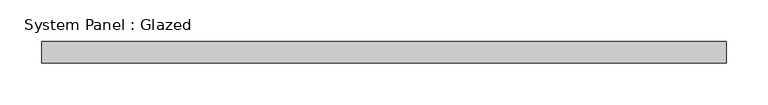
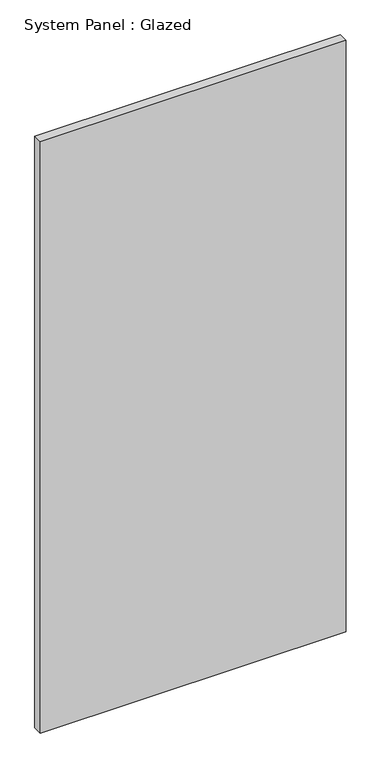
"""IFC4 building model written with IfcOpenShell, lengths in millimetres: plate geometry, System Panel : Glazed."""

from ifc_helpers import new_model, si_unit, origin, origin_with_axes, place, context, project, spatial, polyline, outline, extrude, source, transform, mapped, element, save


def system_panel_glazed_f90b12a9(model_context):
    return source(origin(), model_context, "Body", "SweptSolid", [
        extrude(outline(polyline([(409.575, 19.05), (-409.575, 19.05), (-409.575, 44.45), (409.575, 44.45), (409.575, 19.05)])), origin_with_axes(), (0.0, 0.0, 1.0), 1674.1599467),
    ])


if __name__ == "__main__":
    model = new_model("IFC4")
    model_context = context("Model", 3, world=origin())
    ifc_project = project(units=[si_unit("LENGTHUNIT", "METRE", prefix="MILLI")], contexts=[model_context])
    site = spatial("IfcSite", under=ifc_project)
    building = spatial("IfcBuilding", under=site)
    placement = place(None, origin())
    system_panel_glazed_shape = system_panel_glazed_f90b12a9(model_context)
    element("IfcPlate", 1, ObjectType="System Panel : Glazed", at=placement, inside=building, context=model_context, shape_type="MappedRepresentation", body=[
        mapped(system_panel_glazed_shape, transform((0.0, 0.0, 0.0), x_axis=(1.0, 0.0, 0.0), y_axis=(0.0, 1.0, 0.0), z_axis=(0.0, 0.0, 1.0))),
    ])
    save(model, "model.ifc")

# Revit data of these elements
# Type "System Panel : Glazed"
#   Construction Type Id = "GSP4R"
#   Analytic Construction = "1/8 in Pilkington single glazing"
#   Visual Light Transmittance = 0.9
#   Solar Heat Gain Coefficient = 0.86
#   Heat Transfer Coefficient (U) = 1.18115 BTU/(h·ft²·°F)
#   Define Thermal Properties by = 1
# Element 1 (IfcPlate, "System Panel : Glazed")
#   Materials on its faces: "Glass"
# Materials
#   "Glass": class "Glass", colour RGB 0 128 192, transparency 0.75, Description = "Soda Lime Glass", Cost = 0
